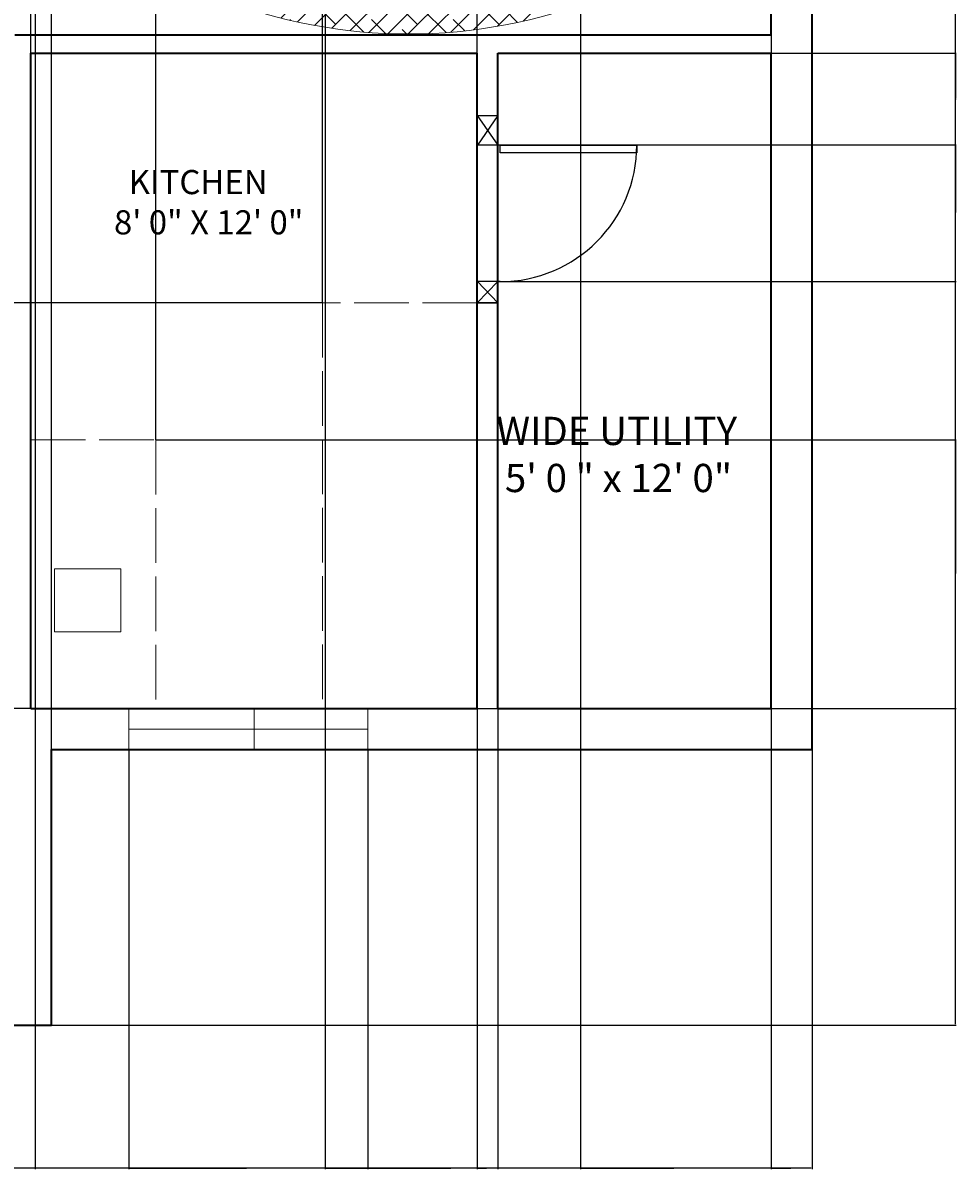
# Model space of a CAD drawing. Units: inches. Extents: x 2284228 to 3635239, y 3024422 to 8351872.
# Tile 3 of 7: x 3635034 to 3635239, y 8351218 to 8351470. Entities that reach past the tile are written whole.
import ezdxf

# ---------------------------------------------------------------- set-up
doc = ezdxf.new("R2010")
doc.units = ezdxf.units.IN
doc.linetypes.add('ACAD_ISO02W100', pattern=[15, 12, -3])
for name, color, linetype, lineweight in [('A-ANNO-DIMS', 2, 'Continuous', 18), ('A-AREA-IDEN', 7, 'Continuous', 18), ('A-DOOR', 4, 'Continuous', 25), ('A-FLOR-CASE-HIDN', 9, 'ACAD_ISO02W100', 18), ('A-FLOR-FIXT', 9, 'Continuous', 18), ('A-FURN', 8, 'Continuous', 18), ('A-FURN-PATT', 9, 'Continuous', 13), ('A-GLAZ', 4, 'Continuous', 18), ('A-WALL', 7, 'Continuous', 35)]:
    doc.layers.add(name, color=color, linetype=linetype, lineweight=lineweight)
doc.styles.get("Standard").update_dxf_attribs({"font": 'arial.ttf'})
doc.dimstyles.get("Standard").update_dxf_attribs({"dimtxt": 0.18, "dimasz": 0.18, "dimexe": 0.18, "dimexo": 0.0625, "dimgap": 0.09, "dimtad": 0, "dimtih": 1, "dimtoh": 1, "dimdec": 4, "dimzin": 0, "dimdsep": 46, "dimtxsty": 'Standard', "dimcen": 0.09, "dimadec": 0, "dimazin": 0, "dimtfac": 1, "dimtdec": 4, "dimtofl": 0, "dimtmove": 0, "dimatfit": 3, "dimfxl": 1, "dimtolj": 1, "dimtzin": 0, "dimarcsym": 0})

# ---------------------------------------------------------------- blocks, each defined once
blk = doc.blocks.new('*U11')
for p, q in [((0, 0), (0, -5)), ((30, 0), (30, -5))]:
    blk.add_line(p, q)
blk.add_lwpolyline([(0, 0), (0, 30), (1.75, 30), (1.75, 0)], close=True)
blk.add_arc((0, 0), 30, 0, 90)
blk = doc.blocks.new('Sofa - Roundback 7 ft.')
for p, q in [((-12.00002, -32.4421), (-12.00003, -6.5971)), ((11.99997, -32.4421), (11.99998, -6.5971)), ((-36.000027, -34), (-36.000027, -11.4696)), ((35.99998, -34), (35.99998, -11.4696)), ((-35.999844, -13.3819), (35.9998, -13.3819)), ((-36.000027, -32.4421), (35.99998, -32.4421))]:
    blk.add_line(p, q)
for points in [[(-36.000027, -34), (-42.000027, -34), (-42.000027, -8)], [(41.99998, -8), (41.99998, -34), (35.99998, -34)]]:
    blk.add_lwpolyline(points)
for centre, radius, start, end in [((0, -114.25), 114.25, 68.43141, 111.5686), ((-0.00001, -127.1968), 121.1968, 72.72033, 107.2797)]:
    blk.add_arc(centre, radius, start, end)
blk = doc.blocks.new('*D40')
at = {"layer": 'A-ANNO-DIMS', "color": 0, "lineweight": -2, "transparency": 16777216}
for p, q in [((3634700.92, 8351463.5), (3634700.92, 8351218.43)), ((3635206.75, 8351310.5), (3635206.75, 8351218.43)), ((3634701.1, 8351218.61), (3634953.44, 8351218.61)), ((3635206.57, 8351218.61), (3634954.23, 8351218.61))]:
    blk.add_line(p, q, dxfattribs=at)
at = {"layer": 'A-ANNO-DIMS', "color": 0, "transparency": 16777216}
for points in [[(3634701.1, 8351218.64), (3634701.1, 8351218.58), (3634700.92, 8351218.61)], [(3635206.57, 8351218.64), (3635206.57, 8351218.58), (3635206.75, 8351218.61)]]:
    blk.add_solid(points, dxfattribs=at)
at = {"layer": 'Defpoints', "color": 0, "transparency": 16777216}
for p in [(3634700.92, 8351463.56), (3635206.75, 8351310.56), (3635206.75, 8351218.61)]:
    blk.add_point(p, dxfattribs=at)
at = {"layer": 'A-ANNO-DIMS', "color": 0, "transparency": 16777216, "insert": (3634953.83, 8351218.61), "char_height": 0.18, "attachment_point": 5}
blk.add_mtext('\\A1;505.8', dxfattribs=at)
blk = doc.blocks.new('*D41')
at = {"layer": 'A-ANNO-DIMS', "color": 0, "lineweight": -2, "transparency": 16777216}
for p, q in [((3635053.81, 8351799.01), (3635238.38, 8351799.01)), ((3635238.2, 8351798.83), (3635238.2, 8351524.72)), ((3635238.2, 8351250.24), (3635238.2, 8351524.36)), ((3635039.81, 8351250.06), (3635238.38, 8351250.06))]:
    blk.add_line(p, q, dxfattribs=at)
at = {"layer": 'A-ANNO-DIMS', "color": 0, "transparency": 16777216}
for points in [[(3635238.17, 8351798.83), (3635238.23, 8351798.83), (3635238.2, 8351799.01)], [(3635238.17, 8351250.24), (3635238.23, 8351250.24), (3635238.2, 8351250.06)]]:
    blk.add_solid(points, dxfattribs=at)
at = {"layer": 'Defpoints', "color": 0, "transparency": 16777216}
for p in [(3635053.75, 8351799.01), (3635238.2, 8351799.01), (3635039.75, 8351250.06)]:
    blk.add_point(p, dxfattribs=at)
at = {"layer": 'A-ANNO-DIMS', "color": 0, "transparency": 16777216, "insert": (3635238.2, 8351524.54), "char_height": 0.18, "attachment_point": 5}
blk.add_mtext('\\A1;549', dxfattribs=at)
blk = doc.blocks.new('*D49')
at = {"layer": 'A-ANNO-DIMS', "color": 0, "lineweight": -2, "transparency": 16777216}
for p, q in [((3634891.75, 8351310.63), (3634891.75, 8351830.64)), ((3634891.93, 8351830.46), (3634965.47, 8351830.46)), ((3635039.57, 8351830.46), (3634966.03, 8351830.46)), ((3635039.75, 8351310.63), (3635039.75, 8351830.64))]:
    blk.add_line(p, q, dxfattribs=at)
at = {"layer": 'A-ANNO-DIMS', "color": 0, "transparency": 16777216}
for points in [[(3634891.93, 8351830.49), (3634891.93, 8351830.43), (3634891.75, 8351830.46)], [(3635039.57, 8351830.49), (3635039.57, 8351830.43), (3635039.75, 8351830.46)]]:
    blk.add_solid(points, dxfattribs=at)
at = {"layer": 'Defpoints', "color": 0, "transparency": 16777216}
for p in [(3635039.75, 8351830.46), (3634891.75, 8351310.56), (3635039.75, 8351310.56)]:
    blk.add_point(p, dxfattribs=at)
at = {"layer": 'A-ANNO-DIMS', "color": 0, "transparency": 16777216, "insert": (3634965.75, 8351830.46), "char_height": 0.18, "attachment_point": 5}
blk.add_mtext('\\A1;148', dxfattribs=at)
blk = doc.blocks.new('*D52')
at = {"layer": 'A-ANNO-DIMS', "color": 0, "lineweight": -2, "transparency": 16777216}
for p, q in [((3635099.83, 8351748.5), (3635099.83, 8351218.43)), ((3635155.88, 8351748.5), (3635155.88, 8351218.43)), ((3635100.01, 8351218.61), (3635127.46, 8351218.61)), ((3635155.7, 8351218.61), (3635128.25, 8351218.61))]:
    blk.add_line(p, q, dxfattribs=at)
at = {"layer": 'A-ANNO-DIMS', "color": 0, "transparency": 16777216}
for points in [[(3635100.01, 8351218.64), (3635100.01, 8351218.58), (3635099.83, 8351218.61)], [(3635155.7, 8351218.64), (3635155.7, 8351218.58), (3635155.88, 8351218.61)]]:
    blk.add_solid(points, dxfattribs=at)
at = {"layer": 'Defpoints', "color": 0, "transparency": 16777216}
for p in [(3635099.83, 8351748.56), (3635155.88, 8351748.56), (3635155.88, 8351218.61)]:
    blk.add_point(p, dxfattribs=at)
at = {"layer": 'A-ANNO-DIMS', "color": 0, "transparency": 16777216, "insert": (3635127.85, 8351218.61), "char_height": 0.18, "attachment_point": 5}
blk.add_mtext('\\A1;56.06', dxfattribs=at)
blk = doc.blocks.new('*D53')
at = {"layer": 'A-ANNO-DIMS', "color": 0, "lineweight": -2, "transparency": 16777216}
for p, q in [((3635155.88, 8351748.5), (3635155.88, 8351218.43)), ((3635197.75, 8351748.5), (3635197.75, 8351218.43)), ((3635156.06, 8351218.61), (3635176.42, 8351218.61)), ((3635197.57, 8351218.61), (3635177.21, 8351218.61))]:
    blk.add_line(p, q, dxfattribs=at)
at = {"layer": 'A-ANNO-DIMS', "color": 0, "transparency": 16777216}
for points in [[(3635156.06, 8351218.64), (3635156.06, 8351218.58), (3635155.88, 8351218.61)], [(3635197.57, 8351218.64), (3635197.57, 8351218.58), (3635197.75, 8351218.61)]]:
    blk.add_solid(points, dxfattribs=at)
at = {"layer": 'Defpoints', "color": 0, "transparency": 16777216}
for p in [(3635155.88, 8351748.56), (3635197.75, 8351748.56), (3635197.75, 8351218.61)]:
    blk.add_point(p, dxfattribs=at)
at = {"layer": 'A-ANNO-DIMS', "color": 0, "transparency": 16777216, "insert": (3635176.82, 8351218.61), "char_height": 0.18, "attachment_point": 5}
blk.add_mtext('\\A1;41.87', dxfattribs=at)
blk = doc.blocks.new('*D54')
at = {"layer": 'A-ANNO-DIMS', "color": 0, "lineweight": -2, "transparency": 16777216}
for p, q in [((3635006.17, 8351652.5), (3635006.17, 8351218.43)), ((3635036.17, 8351652.5), (3635036.17, 8351218.43)), ((3635006.35, 8351218.61), (3635020.95, 8351218.61)), ((3635035.99, 8351218.61), (3635021.38, 8351218.61))]:
    blk.add_line(p, q, dxfattribs=at)
at = {"layer": 'A-ANNO-DIMS', "color": 0, "transparency": 16777216}
for points in [[(3635006.35, 8351218.64), (3635006.35, 8351218.58), (3635006.17, 8351218.61)], [(3635035.99, 8351218.64), (3635035.99, 8351218.58), (3635036.17, 8351218.61)]]:
    blk.add_solid(points, dxfattribs=at)
at = {"layer": 'Defpoints', "color": 0, "transparency": 16777216}
for p in [(3635006.17, 8351652.56), (3635036.17, 8351652.56), (3635036.17, 8351218.61)]:
    blk.add_point(p, dxfattribs=at)
at = {"layer": 'A-ANNO-DIMS', "color": 0, "transparency": 16777216, "insert": (3635021.17, 8351218.61), "char_height": 0.18, "attachment_point": 5}
blk.add_mtext('\\A1;30', dxfattribs=at)
blk = doc.blocks.new('*D56')
at = {"layer": 'A-ANNO-DIMS', "color": 0, "lineweight": -2, "transparency": 16777216}
for p, q in [((3635056.73, 8351310.5), (3635056.73, 8351218.43)), ((3635109.19, 8351310.5), (3635109.19, 8351218.43)), ((3635056.91, 8351218.61), (3635082.57, 8351218.61)), ((3635109.01, 8351218.61), (3635083.35, 8351218.61))]:
    blk.add_line(p, q, dxfattribs=at)
at = {"layer": 'A-ANNO-DIMS', "color": 0, "transparency": 16777216}
for points in [[(3635056.91, 8351218.64), (3635056.91, 8351218.58), (3635056.73, 8351218.61)], [(3635109.01, 8351218.64), (3635109.01, 8351218.58), (3635109.19, 8351218.61)]]:
    blk.add_solid(points, dxfattribs=at)
at = {"layer": 'Defpoints', "color": 0, "transparency": 16777216}
for p in [(3635056.73, 8351310.56), (3635109.19, 8351310.56), (3635109.19, 8351218.61)]:
    blk.add_point(p, dxfattribs=at)
at = {"layer": 'A-ANNO-DIMS', "color": 0, "transparency": 16777216, "insert": (3635082.96, 8351218.61), "char_height": 0.18, "attachment_point": 5}
blk.add_mtext('\\A1;52.46', dxfattribs=at)
blk = doc.blocks.new('*D57')
at = {"layer": 'A-ANNO-DIMS', "color": 0, "lineweight": -2, "transparency": 16777216}
for p, q in [((3635035.25, 8351378.63), (3635035.25, 8351830.64)), ((3635035.43, 8351830.46), (3635048.63, 8351830.46)), ((3635062.47, 8351830.46), (3635049.28, 8351830.46)), ((3635062.65, 8351378.63), (3635062.65, 8351830.64))]:
    blk.add_line(p, q, dxfattribs=at)
at = {"layer": 'A-ANNO-DIMS', "color": 0, "transparency": 16777216}
for points in [[(3635035.43, 8351830.49), (3635035.43, 8351830.43), (3635035.25, 8351830.46)], [(3635062.47, 8351830.49), (3635062.47, 8351830.43), (3635062.65, 8351830.46)]]:
    blk.add_solid(points, dxfattribs=at)
at = {"layer": 'Defpoints', "color": 0, "transparency": 16777216}
for p in [(3635062.65, 8351830.46), (3635035.25, 8351378.57), (3635062.65, 8351378.57)]:
    blk.add_point(p, dxfattribs=at)
at = {"layer": 'A-ANNO-DIMS', "color": 0, "transparency": 16777216, "insert": (3635048.95, 8351830.46), "char_height": 0.18, "attachment_point": 5}
blk.add_mtext('\\A1;27.4', dxfattribs=at)
blk = doc.blocks.new('*D58')
at = {"layer": 'A-ANNO-DIMS', "color": 0, "lineweight": -2, "transparency": 16777216}
for p, q in [((3635062.71, 8351378.57), (3635238.38, 8351378.57)), ((3635238.2, 8351378.39), (3635238.2, 8351349.25)), ((3635238.2, 8351319.74), (3635238.2, 8351348.88)), ((3635062.71, 8351319.56), (3635238.38, 8351319.56))]:
    blk.add_line(p, q, dxfattribs=at)
at = {"layer": 'A-ANNO-DIMS', "color": 0, "transparency": 16777216}
for points in [[(3635238.17, 8351378.39), (3635238.23, 8351378.39), (3635238.2, 8351378.57)], [(3635238.17, 8351319.74), (3635238.23, 8351319.74), (3635238.2, 8351319.56)]]:
    blk.add_solid(points, dxfattribs=at)
at = {"layer": 'Defpoints', "color": 0, "transparency": 16777216}
for p in [(3635062.65, 8351378.57), (3635062.65, 8351319.56), (3635238.2, 8351319.56)]:
    blk.add_point(p, dxfattribs=at)
at = {"layer": 'A-ANNO-DIMS', "color": 0, "transparency": 16777216, "insert": (3635238.2, 8351349.06), "char_height": 0.18, "attachment_point": 5}
blk.add_mtext('\\A1;59', dxfattribs=at)
blk = doc.blocks.new('*D59')
at = {"layer": 'A-ANNO-DIMS', "color": 0, "lineweight": -2, "transparency": 16777216}
for p, q in [((3635099.24, 8351408.73), (3635099.24, 8351830.64)), ((3635099.42, 8351830.46), (3635115.78, 8351830.46)), ((3635133.07, 8351830.46), (3635116.71, 8351830.46)), ((3635133.25, 8351408.73), (3635133.25, 8351830.64))]:
    blk.add_line(p, q, dxfattribs=at)
at = {"layer": 'A-ANNO-DIMS', "color": 0, "transparency": 16777216}
for points in [[(3635099.42, 8351830.49), (3635099.42, 8351830.43), (3635099.24, 8351830.46)], [(3635133.07, 8351830.49), (3635133.07, 8351830.43), (3635133.25, 8351830.46)]]:
    blk.add_solid(points, dxfattribs=at)
at = {"layer": 'Defpoints', "color": 0, "transparency": 16777216}
for p in [(3635133.25, 8351830.46), (3635099.24, 8351408.67), (3635133.25, 8351408.67)]:
    blk.add_point(p, dxfattribs=at)
at = {"layer": 'A-ANNO-DIMS', "color": 0, "transparency": 16777216, "insert": (3635116.24, 8351830.46), "char_height": 0.18, "attachment_point": 5}
blk.add_mtext('\\A1;34.016', dxfattribs=at)
blk = doc.blocks.new('*D60')
at = {"layer": 'A-ANNO-DIMS', "color": 0, "lineweight": -2, "transparency": 16777216}
for p, q in [((3635099.17, 8351408.67), (3634669.29, 8351408.67)), ((3634669.47, 8351408.49), (3634669.47, 8351364.3)), ((3634669.47, 8351319.74), (3634669.47, 8351363.93)), ((3635099.17, 8351319.56), (3634669.29, 8351319.56))]:
    blk.add_line(p, q, dxfattribs=at)
at = {"layer": 'A-ANNO-DIMS', "color": 0, "transparency": 16777216}
for points in [[(3634669.44, 8351408.49), (3634669.5, 8351408.49), (3634669.47, 8351408.67)], [(3634669.44, 8351319.74), (3634669.5, 8351319.74), (3634669.47, 8351319.56)]]:
    blk.add_solid(points, dxfattribs=at)
at = {"layer": 'Defpoints', "color": 0, "transparency": 16777216}
for p in [(3635099.24, 8351408.67), (3634669.47, 8351319.56), (3635099.24, 8351319.56)]:
    blk.add_point(p, dxfattribs=at)
at = {"layer": 'A-ANNO-DIMS', "color": 0, "transparency": 16777216, "insert": (3634669.47, 8351364.12), "char_height": 0.18, "attachment_point": 5}
blk.add_mtext('\\A1;89.1', dxfattribs=at)
blk = doc.blocks.new('*D61')
at = {"layer": 'A-ANNO-DIMS', "color": 0, "lineweight": -2, "transparency": 16777216}
for p, q in [((3635137.81, 8351443.36), (3635238.38, 8351443.36)), ((3635238.2, 8351443.18), (3635238.2, 8351428.54)), ((3635238.2, 8351413.54), (3635238.2, 8351428.18)), ((3635137.81, 8351413.36), (3635238.38, 8351413.36))]:
    blk.add_line(p, q, dxfattribs=at)
at = {"layer": 'A-ANNO-DIMS', "color": 0, "transparency": 16777216}
for points in [[(3635238.17, 8351443.18), (3635238.23, 8351443.18), (3635238.2, 8351443.36)], [(3635238.17, 8351413.54), (3635238.23, 8351413.54), (3635238.2, 8351413.36)]]:
    blk.add_solid(points, dxfattribs=at)
at = {"layer": 'Defpoints', "color": 0, "transparency": 16777216}
for p in [(3635137.75, 8351443.36), (3635238.2, 8351443.36), (3635137.75, 8351413.36)]:
    blk.add_point(p, dxfattribs=at)
at = {"layer": 'A-ANNO-DIMS', "color": 0, "transparency": 16777216, "insert": (3635238.2, 8351428.36), "char_height": 0.18, "attachment_point": 5}
blk.add_mtext('\\A1;30', dxfattribs=at)
blk = doc.blocks.new('*D62')
at = {"layer": 'A-ANNO-DIMS', "color": 0, "lineweight": -2, "transparency": 16777216}
for p, q in [((3635137.81, 8351463.56), (3635238.38, 8351463.56)), ((3635238.2, 8351463.38), (3635238.2, 8351453.64)), ((3635238.2, 8351443.54), (3635238.2, 8351453.28)), ((3635137.81, 8351443.36), (3635238.38, 8351443.36))]:
    blk.add_line(p, q, dxfattribs=at)
at = {"layer": 'A-ANNO-DIMS', "color": 0, "transparency": 16777216}
for points in [[(3635238.17, 8351463.38), (3635238.23, 8351463.38), (3635238.2, 8351463.56)], [(3635238.17, 8351443.54), (3635238.23, 8351443.54), (3635238.2, 8351443.36)]]:
    blk.add_solid(points, dxfattribs=at)
at = {"layer": 'Defpoints', "color": 0, "transparency": 16777216}
for p in [(3635137.75, 8351463.56), (3635238.2, 8351463.56), (3635137.75, 8351443.36)]:
    blk.add_point(p, dxfattribs=at)
at = {"layer": 'A-ANNO-DIMS', "color": 0, "transparency": 16777216, "insert": (3635238.2, 8351453.46), "char_height": 0.18, "attachment_point": 5}
blk.add_mtext('\\A1;20.204', dxfattribs=at)
blk = doc.blocks.new('*D63')
at = {"layer": 'A-ANNO-DIMS', "color": 0, "lineweight": -2, "transparency": 16777216}
for p, q in [((3635197.75, 8351319.5), (3635197.75, 8351218.43)), ((3635206.75, 8351310.5), (3635206.75, 8351218.43)), ((3635197.93, 8351218.61), (3635202.1, 8351218.61)), ((3635206.57, 8351218.61), (3635202.4, 8351218.61))]:
    blk.add_line(p, q, dxfattribs=at)
at = {"layer": 'A-ANNO-DIMS', "color": 0, "transparency": 16777216}
for points in [[(3635197.93, 8351218.64), (3635197.93, 8351218.58), (3635197.75, 8351218.61)], [(3635206.57, 8351218.64), (3635206.57, 8351218.58), (3635206.75, 8351218.61)]]:
    blk.add_solid(points, dxfattribs=at)
at = {"layer": 'Defpoints', "color": 0, "transparency": 16777216}
for p in [(3635197.75, 8351319.56), (3635206.75, 8351310.56), (3635206.75, 8351218.61)]:
    blk.add_point(p, dxfattribs=at)
at = {"layer": 'A-ANNO-DIMS', "color": 0, "transparency": 16777216, "insert": (3635202.25, 8351218.61), "char_height": 0.18, "attachment_point": 5}
blk.add_mtext('\\A1;9', dxfattribs=at)
blk = doc.blocks.new('*D64')
at = {"layer": 'A-ANNO-DIMS', "color": 0, "lineweight": -2, "transparency": 16777216}
for p, q in [((3635133.25, 8351319.5), (3635133.25, 8351218.43)), ((3635137.75, 8351319.5), (3635137.75, 8351218.43)), ((3635133.43, 8351218.61), (3635135.24, 8351218.61)), ((3635137.57, 8351218.61), (3635135.76, 8351218.61))]:
    blk.add_line(p, q, dxfattribs=at)
at = {"layer": 'A-ANNO-DIMS', "color": 0, "transparency": 16777216}
for points in [[(3635133.43, 8351218.64), (3635133.43, 8351218.58), (3635133.25, 8351218.61)], [(3635137.57, 8351218.64), (3635137.57, 8351218.58), (3635137.75, 8351218.61)]]:
    blk.add_solid(points, dxfattribs=at)
at = {"layer": 'Defpoints', "color": 0, "transparency": 16777216}
for p in [(3635133.25, 8351319.56), (3635137.75, 8351319.56), (3635137.75, 8351218.61)]:
    blk.add_point(p, dxfattribs=at)
at = {"layer": 'A-ANNO-DIMS', "color": 0, "transparency": 16777216, "insert": (3635135.5, 8351218.61), "char_height": 0.18, "attachment_point": 5}
blk.add_mtext('\\A1;4.5', dxfattribs=at)

msp = doc.modelspace()

# ---------------------------------------------------------------- hatches: boundary and pattern name
at = {"layer": 'A-FURN-PATT'}
h = msp.add_hatch(dxfattribs=at)
h.set_pattern_fill('ANSI38', color=256)
h.paths.add_polyline_path([(3634930.7271, 8351308.1081), (3634917.6211, 8351308.1081), (3634917.6211, 8351291.6054), (3634930.7271, 8351291.6054)], flags=17)
h.paths.add_polyline_path([(3634917.6211, 8351308.1081), (3634916.3066, 8351308.1081, 0.11251889), (3634912.5453, 8351291.6054), (3634917.6211, 8351291.6054)], flags=17)
h.paths.add_polyline_path([(3634930.7271, 8351291.6054), (3634917.6211, 8351291.6054), (3634917.6211, 8351275.1027), (3634930.7271, 8351275.1027)], flags=17)
h.paths.add_polyline_path([(3634917.6211, 8351291.6054), (3634912.5453, 8351291.6054, 0.11251869), (3634916.3066, 8351275.1027), (3634917.6211, 8351275.1027)], flags=17)
h.paths.add_polyline_path([(3634931.7984, 8351312.2337), (3634913.9206, 8351312.2337, 0.26666697), (3634913.9206, 8351270.977), (3634931.7984, 8351270.977), (3634931.7984, 8351275.1027), (3634916.3066, 8351275.1027, -0.11251869), (3634912.5453, 8351291.6054, -0.11251889), (3634916.3066, 8351308.1081), (3634931.7984, 8351308.1081)])
h.paths.add_polyline_path([(3635011.8389, 8351305.2814), (3634998.7329, 8351305.2814), (3634998.7329, 8351288.7787), (3635011.8389, 8351288.7787)], flags=17)
h.paths.add_polyline_path([(3635011.8389, 8351288.7787), (3634998.7329, 8351288.7787), (3634998.7329, 8351272.276), (3635011.8389, 8351272.276)], flags=17)
h.paths.add_polyline_path([(3635016.9148, 8351288.7787), (3635011.8389, 8351288.7787), (3635011.8389, 8351272.276), (3635013.1534, 8351272.276, 0.11251889)], flags=17)
h.paths.add_polyline_path([(3635013.1534, 8351305.2814), (3635011.8389, 8351305.2814), (3635011.8389, 8351288.7787), (3635016.9148, 8351288.7787, 0.11251869)], flags=17)
h.paths.add_polyline_path([(3635015.5395, 8351309.407), (3634997.6616, 8351309.407), (3634997.6616, 8351305.2814), (3635013.1534, 8351305.2814, -0.11251869), (3635016.9148, 8351288.7787, -0.11251889), (3635013.1534, 8351272.276), (3634997.6616, 8351272.276), (3634997.6616, 8351268.1503), (3635015.5395, 8351268.1503, 0.26666697)])
h.paths.add_polyline_path([(3635065.1595, 8351552.9755), (3635052.0535, 8351552.9755), (3635052.0535, 8351536.4728), (3635065.1595, 8351536.4728)], flags=17)
h.paths.add_polyline_path([(3635065.1595, 8351536.4728), (3635052.0535, 8351536.4728), (3635052.0535, 8351519.9701), (3635065.1595, 8351519.9701)], flags=17)
h.paths.add_polyline_path([(3635052.0535, 8351536.4728), (3635046.9776, 8351536.4728, 0.11251869), (3635050.739, 8351519.9701), (3635052.0535, 8351519.9701)], flags=17)
h.paths.add_polyline_path([(3635052.0535, 8351552.9755), (3635050.739, 8351552.9755, 0.11251889), (3635046.9776, 8351536.4728), (3635052.0535, 8351536.4728)], flags=17)
h.paths.add_polyline_path([(3635066.2308, 8351519.9701), (3635050.739, 8351519.9701, -0.11251869), (3635046.9776, 8351536.4728, -0.11251889), (3635050.739, 8351552.9755), (3635066.2308, 8351552.9755), (3635066.2308, 8351557.1011), (3635048.3529, 8351557.1011, 0.26666697), (3635048.3529, 8351515.8444), (3635066.2308, 8351515.8444)])
h.paths.add_polyline_path([(3635177.7039, 8351552.9754), (3635164.5979, 8351552.9754), (3635164.5979, 8351536.4728), (3635177.7039, 8351536.4728)], flags=17)
h.paths.add_polyline_path([(3635179.0184, 8351552.9754), (3635177.7039, 8351552.9754), (3635177.7039, 8351536.4728), (3635182.7797, 8351536.4728, 0.11251869)], flags=17)
h.paths.add_polyline_path([(3635177.7039, 8351536.4728), (3635164.5979, 8351536.4728), (3635164.5979, 8351519.9701), (3635177.7039, 8351519.9701)], flags=17)
h.paths.add_polyline_path([(3635182.7797, 8351536.4728), (3635177.7039, 8351536.4728), (3635177.7039, 8351519.9701), (3635179.0184, 8351519.9701, 0.11251889)], flags=17)
h.paths.add_polyline_path([(3635181.4045, 8351557.1011), (3635163.5266, 8351557.1011), (3635163.5266, 8351552.9754), (3635179.0184, 8351552.9754, -0.11251869), (3635182.7797, 8351536.4728, -0.11251889), (3635179.0184, 8351519.9701), (3635163.5266, 8351519.9701), (3635163.5266, 8351515.8444), (3635181.4045, 8351515.8444, 0.26666697)])
h.paths.add_polyline_path([(3635154.1523, 8351500.1911), (3635130.1523, 8351500.1911), (3635130.1523, 8351481.1309), (3635154.1523, 8351481.1309)], flags=17)
h.paths.add_polyline_path([(3635130.1523, 8351500.1911), (3635106.1523, 8351500.1911), (3635106.1523, 8351481.1309), (3635130.1523, 8351481.1309)], flags=17)
h.paths.add_polyline_path([(3635106.1523, 8351500.1911), (3635082.1523, 8351500.1911), (3635082.1523, 8351481.1309), (3635106.1523, 8351481.1309)], flags=17)
h.paths.add_polyline_path([(3635106.1523, 8351481.1309), (3635082.1523, 8351481.1309), (3635082.1523, 8351479.2191, 0.05064665), (3635106.1523, 8351474.3445)], flags=17)
h.paths.add_polyline_path([(3635130.1523, 8351481.1309), (3635106.1523, 8351481.1309), (3635106.1523, 8351474.3461), (3635106.1523, 8351474.3445, 0.04962821), (3635130.1523, 8351474.3445)], flags=17)
h.paths.add_polyline_path([(3635154.1523, 8351479.2191), (3635154.1523, 8351481.1309), (3635130.1523, 8351481.1309), (3635130.1523, 8351474.3445, 0.05064665)], flags=17)
h.paths.add_polyline_path([(3635160.1523, 8351475.749), (3635160.1523, 8351501.749), (3635154.1523, 8351501.749), (3635154.1523, 8351479.2191, -0.15194781), (3635082.1523, 8351479.2191), (3635082.1523, 8351501.749), (3635076.1523, 8351501.749), (3635076.1523, 8351475.749, 0.19047621)])

# ---------------------------------------------------------------- linework, layer by layer
at = {"layer": 'A-DOOR'}
for p, q in [((3635133.2525, 8351449.8594), (3635137.7525, 8351449.8594)), ((3635133.2525, 8351449.8594), (3635137.7525, 8351443.3583)), ((3635137.7525, 8351449.8594), (3635133.2773, 8351443.3583)), ((3635137.7525, 8351443.3583), (3635137.7525, 8351449.8594)), ((3635133.2525, 8351408.6677), (3635137.7525, 8351413.3583)), ((3635133.2773, 8351413.3583), (3635137.7525, 8351408.6677)), ((3635133.2525, 8351408.6677), (3635137.7525, 8351408.6677)), ((3635137.7525, 8351408.6677), (3635133.2525, 8351408.6677))]:
    msp.add_line(p, q, dxfattribs=at)
at = {"layer": 'A-FLOR-CASE-HIDN'}
for p, q in [((3635133.2525, 8351408.6677), (3635099.2364, 8351408.6677)), ((3635099.2364, 8351408.6677), (3635099.2364, 8351319.5627)), ((3635035.2525, 8351378.5661), (3635062.6524, 8351378.5661)), ((3635062.6524, 8351378.5661), (3635062.6524, 8351319.5627))]:
    msp.add_line(p, q, dxfattribs=at)
at = {"layer": 'A-FLOR-FIXT'}
for p, q in [((3635040.4436, 8351350.2625), (3635054.9679, 8351350.2625)), ((3635040.4436, 8351350.2625), (3635040.4436, 8351336.432)), ((3635054.9679, 8351350.2625), (3635054.9679, 8351336.432)), ((3635054.9679, 8351336.432), (3635040.4436, 8351336.432))]:
    msp.add_line(p, q, dxfattribs=at)
at = {"layer": 'A-GLAZ'}
for p, q in [((3635056.7309, 8351319.5627), (3635056.7309, 8351310.5627)), ((3635084.2525, 8351319.5627), (3635084.2525, 8351310.5627)), ((3635109.1874, 8351319.5627), (3635109.1874, 8351310.5627)), ((3635056.7309, 8351315.0627), (3635109.1874, 8351315.0627))]:
    msp.add_line(p, q, dxfattribs=at)
at = {"layer": 'A-WALL'}
for p, q in [((3635206.7525, 8351310.5627), (3635206.7525, 8351757.5627)), ((3635197.7525, 8351467.5627), (3635197.7525, 8351600.0627)), ((3635031.7525, 8351467.5627), (3635197.7525, 8351467.5627)), ((3635035.2525, 8351319.5627), (3635035.2525, 8351463.5627)), ((3635035.2525, 8351463.5627), (3635133.2525, 8351463.5627)), ((3635133.2525, 8351319.5627), (3635133.2525, 8351463.5627)), ((3635137.7525, 8351319.5627), (3635137.7525, 8351463.5627)), ((3635137.7525, 8351463.5627), (3635197.7525, 8351463.5627)), ((3635197.7525, 8351319.5627), (3635197.7525, 8351463.5627)), ((3635035.2525, 8351319.5627), (3635133.2525, 8351319.5627)), ((3635035.2525, 8351319.5627), (3635133.2525, 8351319.5627)), ((3635137.7525, 8351319.5627), (3635197.7525, 8351319.5627)), ((3635137.7525, 8351319.5627), (3635197.7525, 8351319.5627)), ((3635039.7525, 8351310.5627), (3635206.7525, 8351310.5627)), ((3635039.7525, 8351250.0627), (3635039.7525, 8351310.5627)), ((3634891.7525, 8351250.0627), (3635039.7525, 8351250.0627))]:
    msp.add_line(p, q, dxfattribs=at)

# ---------------------------------------------------------------- block references
at = {"layer": 'A-DOOR', "rotation": 270}
msp.add_blockref('*U11', (3635138.2773, 8351443.3583), dxfattribs=at)
at = {"layer": 'A-FURN', "rotation": 180}
msp.add_blockref('Sofa - Roundback 7 ft.', (3635118.1522, 8351467.749), dxfattribs=at)

# ---------------------------------------------------------------- texts
at = {"layer": 'A-AREA-IDEN', "attachment_point": 1}
for s, width, gutter_width, insert, char_height in [('    KITCHEN\\P  8\' 0" X 12\' 0"', 216.217558, 26.5164, (3635050.2445, 8351437.8662), 5.303286), ('      WIDE UTILITY\\P       5\' 0 " x 12\' 0"', 153.899863, 30.9973, (3635126.0466, 8351383.6579), 6.199469)]:
    msp.add_mtext_dynamic_manual_height_columns(s, width=width, gutter_width=gutter_width, heights=[0], dxfattribs=dict(at, insert=insert, char_height=char_height))

# ---------------------------------------------------------------- dimensions: what is measured, and where the dimension line sits
at = {"layer": 'A-ANNO-DIMS'}
for base, p1, p2, override, picture, middle in [((3635039.7525, 8351830.4618), (3634891.7525, 8351310.5627), (3635039.7525, 8351310.5627), {"dimdec": 0, "dimlfac": 1, "dimrnd": 0, "dimzin": 0, "dimdsep": 46, "dimlunit": 2}, '*D49', (3634965.7525, 8351830.4618)), ((3635062.6524, 8351830.4618), (3635035.2525, 8351378.5661), (3635062.6524, 8351378.5661), {"dimdec": 1, "dimlfac": 1, "dimrnd": 0, "dimzin": 0, "dimdsep": 46, "dimlunit": 2}, '*D57', (3635048.9524, 8351830.4618)), ((3635133.2525, 8351830.4618), (3635099.2364, 8351408.6677), (3635133.2525, 8351408.6677), {"dimdec": 3, "dimlfac": 1, "dimrnd": 0, "dimzin": 0, "dimdsep": 46, "dimlunit": 2}, '*D59', (3635116.2444, 8351830.4618)), ((3635155.8817, 8351218.6127), (3635099.8261, 8351748.5627), (3635155.8817, 8351748.5627), {"dimdec": 2, "dimlfac": 1, "dimrnd": 0, "dimzin": 0, "dimdsep": 46, "dimlunit": 2}, '*D52', (3635127.8539, 8351218.6127)), ((3635197.7525, 8351218.6127), (3635155.8817, 8351748.5627), (3635197.7525, 8351748.5627), {"dimdec": 2, "dimlfac": 1, "dimrnd": 0, "dimzin": 0, "dimdsep": 46, "dimlunit": 2}, '*D53', (3635176.8171, 8351218.6127)), ((3635036.1658, 8351218.6127), (3635006.1658, 8351652.5627), (3635036.1658, 8351652.5627), {"dimdec": 0, "dimlfac": 1, "dimrnd": 0, "dimzin": 0, "dimdsep": 46, "dimlunit": 2}, '*D54', (3635021.1658, 8351218.6127)), ((3635206.7525, 8351218.6127), (3634700.915, 8351463.5627), (3635206.7525, 8351310.5627), {"dimdec": 1, "dimlfac": 1, "dimrnd": 0, "dimzin": 0, "dimdsep": 46, "dimlunit": 2}, '*D40', (3634953.8337, 8351218.6127)), ((3635137.7525, 8351218.6127), (3635133.2525, 8351319.5627), (3635137.7525, 8351319.5627), {"dimdec": 1, "dimlfac": 1, "dimrnd": 0, "dimzin": 0, "dimdsep": 46, "dimlunit": 2}, '*D64', (3635135.5025, 8351218.6127)), ((3635206.7525, 8351218.6127), (3635197.7525, 8351319.5627), (3635206.7525, 8351310.5627), {"dimdec": 0, "dimlfac": 1, "dimrnd": 0, "dimzin": 0, "dimdsep": 46, "dimlunit": 2}, '*D63', (3635202.2525, 8351218.6127)), ((3635109.1874, 8351218.6127), (3635056.7309, 8351310.5627), (3635109.1874, 8351310.5627), {"dimdec": 2, "dimlfac": 1, "dimrnd": 0, "dimzin": 0, "dimdsep": 46, "dimlunit": 2}, '*D56', (3635082.9591, 8351218.6127))]:
    dim = msp.add_linear_dim(base=base, p1=p1, p2=p2, dimstyle='Standard', override=override, dxfattribs=at)
    dim.commit()
    dim.dimension.update_dxf_attribs({"geometry": picture, "text_midpoint": middle})
for base, p1, p2, override, picture, middle in [((3635238.2025, 8351799.0118), (3635039.7525, 8351250.0627), (3635053.7525, 8351799.0118), {"dimdec": 0, "dimlfac": 1, "dimrnd": 0, "dimzin": 0, "dimdsep": 46, "dimlunit": 2}, '*D41', (3635238.2025, 8351524.5372)), ((3635238.2025, 8351463.5627), (3635137.7525, 8351443.3583), (3635137.7525, 8351463.5627), {"dimdec": 3, "dimlfac": 1, "dimrnd": 0, "dimzin": 0, "dimdsep": 46, "dimlunit": 2}, '*D62', (3635238.2025, 8351453.4605)), ((3635238.2025, 8351443.3583), (3635137.7525, 8351413.3583), (3635137.7525, 8351443.3583), {"dimdec": 0, "dimlfac": 1, "dimrnd": 0, "dimzin": 0, "dimdsep": 46, "dimlunit": 2}, '*D61', (3635238.2025, 8351428.3583)), ((3634669.465, 8351319.5627), (3635099.2364, 8351408.6677), (3635099.2364, 8351319.5627), {"dimdec": 1, "dimlfac": 1, "dimrnd": 0, "dimzin": 0, "dimdsep": 46, "dimlunit": 2}, '*D60', (3634669.465, 8351364.1152)), ((3635238.2025, 8351319.5627), (3635062.6524, 8351378.5661), (3635062.6524, 8351319.5627), {"dimdec": 0, "dimlfac": 1, "dimrnd": 0, "dimzin": 0, "dimdsep": 46, "dimlunit": 2}, '*D58', (3635238.2025, 8351349.0644))]:
    dim = msp.add_linear_dim(base=base, p1=p1, p2=p2, angle=90, dimstyle='Standard', override=override, dxfattribs=at)
    dim.commit()
    dim.dimension.update_dxf_attribs({"geometry": picture, "text_midpoint": middle})

doc.saveas('drawing.dxf')
